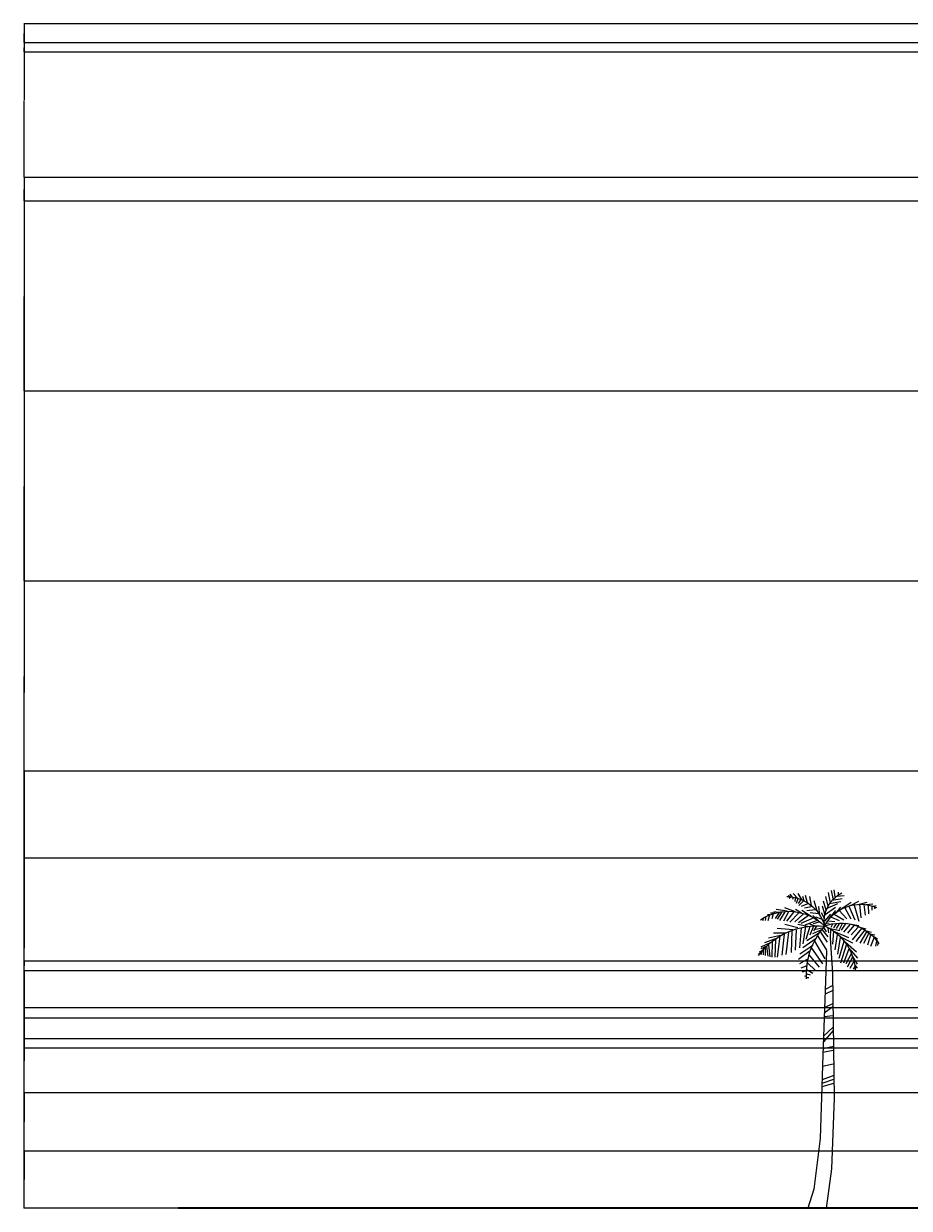
# Model space of a CAD drawing. Units: inches. Extents: x -742 to 1386, y -64 to 951.
# Tile 1 of 8: x -742 to -183, y 106 to 854. Entities that reach past the tile are written whole.
import ezdxf

# ---------------------------------------------------------------- set-up
doc = ezdxf.new("R2010")
doc.units = ezdxf.units.IN
doc.header["$MEASUREMENT"] = 0
for name, color, linetype, lineweight in [('A-ANNO-DIMS', 2, 'Continuous', 18), ('A-ELEV', 7, 'Continuous', 35), ('tree', 3, 'Continuous', 18)]:
    doc.layers.add(name, color=color, linetype=linetype, lineweight=lineweight)
doc.styles.get("Standard").update_dxf_attribs({"font": 'arial.ttf'})
doc.dimstyles.get("Standard").update_dxf_attribs({"dimtxt": 0.18, "dimasz": 0.18, "dimexe": 0.18, "dimexo": 0.0625, "dimgap": 0.09, "dimtad": 0, "dimtih": 1, "dimtoh": 1, "dimdec": 4, "dimzin": 0, "dimdsep": 46, "dimtxsty": 'Standard', "dimcen": 0.09, "dimadec": 0, "dimazin": 0, "dimtfac": 1, "dimtdec": 4, "dimtofl": 0, "dimtmove": 0, "dimatfit": 3, "dimfxl": 1, "dimtolj": 1, "dimtzin": 0, "dimarcsym": 0})

# ---------------------------------------------------------------- blocks, each defined once
blk = doc.blocks.new('*U2')
for p, q in [((-6.727, 197.202), (-11.366, 197.45)), ((-3.441, 194.477), (-10.013, 195.716)), ((-7.5, 199.68), (-7.5, 197.946)), ((-5.567, 196.707), (-4.987, 201.167)), ((-4.407, 195.716), (-3.247, 200.672)), ((-2.474, 193.733), (-1.315, 199.433)), ((-1.121, 190.759), (0.232, 196.955)), ((9.317, 191.255), (10.283, 196.955)), ((11.829, 192.99), (13.182, 197.45)), ((13.956, 194.229), (14.729, 196.955)), ((15.116, 194.477), (17.822, 198.689)), ((16.082, 194.972), (17.822, 192.494)), ((18.015, 195.716), (20.914, 198.689)), ((18.015, 195.468), (18.981, 192.494)), ((19.368, 196.459), (19.948, 193.733)), ((20.914, 196.459), (21.301, 194.972)), ((21.301, 196.459), (22.847, 198.441)), ((22.074, 196.707), (23.427, 195.716)), ((23.234, 196.707), (23.62, 197.698)), ((-29.729, 190.759), (-31.469, 191.255)), ((-30.309, 190.512), (-30.695, 189.025)), ((-25.283, 191.751), (-29.342, 192.246)), ((-28.763, 190.759), (-28.763, 188.281)), ((-26.443, 191.503), (-26.636, 186.051)), ((-20.064, 191.751), (-25.863, 193.238)), ((-23.737, 191.751), (-24.51, 185.06)), ((-21.031, 191.998), (-21.804, 183.325)), ((-15.232, 191.255), (-20.644, 193.981)), ((-17.551, 191.503), (-20.451, 181.343)), ((-14.265, 190.759), (-18.131, 182.086)), ((-9.433, 189.025), (-15.618, 193.238)), ((-11.753, 189.768), (-15.425, 182.83)), ((-8.08, 188.034), (-12.912, 182.83)), ((-1.894, 192.494), (-9.24, 193.733)), ((-6.147, 186.299), (-9.24, 190.264)), ((-0.541, 189.52), (-7.307, 192.494)), ((-5.76, 190.016), (0.618, 185.308)), ((-5.76, 188.034), (-1.508, 182.582)), ((0.038, 188.281), (1.778, 193.981)), ((1.005, 185.803), (2.358, 190.759)), ((4.098, 185.06), (4.678, 190.512)), ((5.837, 187.786), (7.577, 194.229)), ((6.997, 188.529), (12.216, 187.786)), ((8.544, 190.512), (13.763, 189.52)), ((9.51, 184.317), (15.502, 188.034)), ((11.25, 192.494), (15.889, 190.512)), ((14.536, 193.981), (17.242, 191.255)), ((15.695, 186.299), (19.368, 188.777)), ((19.368, 187.29), (26.133, 189.768)), ((20.721, 187.042), (25.167, 181.343)), ((23.814, 187.29), (26.907, 181.343)), ((24.78, 187.538), (31.546, 188.777)), ((26.133, 187.29), (29.419, 181.838)), ((28.066, 187.29), (30.966, 182.582)), ((29.999, 186.795), (33.092, 187.29)), ((-12.332, 180.104), (-9.433, 175.643)), ((-4.987, 185.803), (-10.979, 182.086)), ((-10.206, 180.104), (-8.08, 175.891)), ((-8.273, 180.104), (-6.147, 176.635)), ((-3.247, 183.821), (-8.08, 181.838)), ((-6.34, 179.608), (-4.6, 177.13)), ((-1.315, 181.591), (-5.374, 181.095)), ((-2.668, 185.803), (1.198, 181.343)), ((-0.348, 180.352), (-1.894, 180.104)), ((1.005, 182.582), (2.938, 186.547)), ((2.938, 182.582), (6.61, 183.821)), ((4.098, 180.847), (8.35, 179.608)), ((4.871, 186.051), (10.09, 186.547)), ((4.871, 181.591), (8.544, 184.812)), ((5.644, 181.838), (13.569, 178.865)), ((7.77, 183.325), (16.082, 179.856)), ((11.25, 184.812), (17.628, 180.352)), ((14.536, 185.803), (19.948, 180.847)), ((17.242, 186.547), (23.041, 180.599)), ((29.806, 186.795), (32.319, 183.078)), ((32.512, 186.299), (35.218, 186.299)), ((33.479, 186.051), (34.445, 182.83)), ((35.605, 185.556), (37.151, 185.308)), ((35.798, 185.308), (36.958, 181.591)), ((38.118, 184.317), (38.504, 181.838)), ((39.857, 182.83), (40.244, 181.591)), ((-28.956, 172.174), (-32.435, 170.192)), ((-27.409, 173.413), (-30.695, 172.67)), ((-25.09, 175.148), (-28.376, 174.404)), ((-27.989, 172.422), (-26.056, 166.227)), ((-26.829, 173.661), (-23.544, 167.218)), ((-25.476, 174.652), (-21.224, 167.466)), ((-21.031, 177.626), (-24.897, 176.387)), ((-24.317, 175.891), (-18.711, 168.457)), ((-22.191, 176.635), (-16.391, 169.448)), ((-15.618, 179.36), (-20.644, 178.617)), ((-20.064, 177.626), (-15.812, 172.67)), ((-17.358, 178.617), (-13.299, 173.661)), ((-15.038, 179.36), (-10.786, 174.404)), ((-4.214, 175.148), (-14.072, 170.935)), ((-1.701, 176.882), (-8.66, 175.396)), ((-6.92, 172.917), (-5.374, 163.253)), ((-4.6, 174.9), (-4.021, 166.722)), ((-4.021, 179.36), (-2.861, 177.378)), ((-2.668, 176.387), (-2.376, 170.594)), ((-0.928, 176.882), (-1.508, 173.909)), ((2.551, 175.891), (-0.928, 171.431)), ((3.711, 174.404), (-0.541, 167.961)), ((1.585, 177.13), (0.038, 174.652)), ((1.585, 177.13), (6.61, 176.139)), ((2.938, 175.891), (8.737, 173.413)), ((4.291, 173.909), (12.216, 168.953)), ((6.224, 178.121), (8.157, 175.148)), ((7.384, 178.369), (10.476, 179.36)), ((8.157, 178.121), (10.476, 172.422)), ((10.476, 177.874), (12.796, 169.696)), ((11.829, 177.874), (18.015, 179.113)), ((13.182, 177.874), (14.729, 166.97)), ((15.889, 177.13), (16.855, 164.492)), ((18.015, 177.13), (26.133, 179.113)), ((18.981, 175.891), (19.561, 163.005)), ((20.914, 175.891), (30.966, 176.635)), ((21.688, 175.396), (22.074, 161.518)), ((23.814, 174.404), (25.554, 160.279)), ((25.554, 173.661), (33.285, 173.661)), ((26.52, 173.165), (28.066, 159.784)), ((28.839, 172.174), (36.378, 170.687)), ((-32.628, 167.961), (-33.208, 167.961)), ((-32.628, 167.713), (-32.435, 165.979)), ((-31.082, 169.944), (-32.435, 169.2)), ((-31.662, 168.705), (-31.082, 165.483)), ((-29.922, 170.687), (-27.989, 165.235)), ((-12.139, 167.961), (-19.098, 162.014)), ((-8.466, 171.678), (-16.585, 167.713)), ((-12.719, 166.722), (-9.046, 154.828)), ((-10.979, 168.457), (-7.887, 157.801)), ((-8.853, 170.935), (-7.113, 160.527)), ((5.257, 171.926), (-0.155, 163.005)), ((7.384, 168.705), (0.812, 157.553)), ((6.417, 170.439), (14.729, 164.492)), ((8.544, 165.979), (16.662, 160.527)), ((29.226, 171.926), (30.966, 158.545)), ((30.966, 170.687), (38.891, 167.713)), ((32.126, 169.696), (32.512, 158.545)), ((34.058, 168.705), (34.445, 158.545)), ((35.412, 167.713), (41.404, 164.988)), ((36.378, 166.474), (35.605, 158.792)), ((37.731, 165.235), (36.958, 159.288)), ((37.924, 165.235), (41.404, 163.749)), ((-14.265, 164.244), (-19.678, 158.049)), ((-16.005, 160.031), (-19.484, 154.084)), ((-16.585, 158.545), (-13.106, 152.35)), ((-15.618, 160.775), (-12.332, 154.332)), ((-14.265, 163.749), (-10.786, 154.828)), ((9.317, 164.244), (2.358, 154.332)), ((10.863, 159.784), (4.484, 152.35)), ((10.09, 162.51), (17.435, 157.058)), ((11.443, 157.553), (16.855, 154.332)), ((38.504, 164.492), (38.504, 159.536)), ((39.664, 163.253), (42.37, 161.766)), ((39.857, 162.757), (39.857, 160.031)), ((40.824, 161.766), (41.21, 160.031)), ((41.21, 161.518), (42.757, 160.279)), ((-18.131, 153.589), (-19.484, 151.606)), ((-17.938, 152.597), (-16.972, 151.111)), ((-17.358, 155.819), (-14.845, 151.358)), ((11.829, 155.075), (6.804, 150.119)), ((12.603, 151.111), (8.544, 148.385)), ((12.216, 153.093), (16.082, 151.606)), ((12.603, 149.872), (15.116, 149.128)), ((12.216, 148.137), (10.09, 147.393)), ((12.409, 145.659), (11.056, 145.659)), ((12.409, 146.898), (13.763, 146.402)), ((-4.081, 140.645), (0.753, 138.261)), ((-4.081, 137.547), (0.753, 135.163)), ((-4.081, 129.205), (1.124, 126.821)), ((-4.081, 127.298), (1.31, 123.246)), ((-4.081, 121.578), (1.31, 120.863)), ((-4.453, 112.283), (1.682, 105.133)), ((-4.267, 114.428), (1.682, 108.708)), ((-4.639, 102.273), (1.868, 100.604)), ((-4.453, 99.651), (2.24, 98.459)), ((-4.453, 91.071), (2.426, 89.641)), ((-4.825, 83.921), (2.612, 81.061)), ((-4.639, 81.299), (2.797, 78.916)), ((-4.639, 78.916), (2.797, 76.771))]:
    blk.add_line(p, q)
for points in [[(-2.363, 170.553), (-3.88, 148.505), (-4.988, 69.634), (-3.325, 24.869), (0, 0)], [(-0.116, 162.848), (0.554, 143.532), (2.217, 96.635), (3.88, 44.054), (7.76, 12.079), (11.64, 0)]]:
    blk.add_lwpolyline(points)
for centre, radius, start, end in [((-18.427, 181.448), 19.715, 350.285, 64.11229), ((25.595, 171.567), 25.395, 91.40319, 163.882), ((-21.738, 166.094), 25.899, 27.67115, 112.5305), ((23.687, 155.341), 32.188, 56.19272, 134.3213), ((-9.259, 151.732), 28.386, 68.38311, 147.5322), ((14.394, 148.393), 32.752, 113.7592, 177.4133), ((5.828, 132.718), 45.639, 35.98777, 95.82273), ((-32.8, 147.923), 45.309, 356.1943, 41.37848)]:
    blk.add_arc(centre, radius, start, end)
blk = doc.blocks.new('*D40')
at = {"layer": 'A-ANNO-DIMS', "color": 0, "lineweight": -2, "transparency": 16777216}
for p, q in [((-46.83, 756.74), (-741.55, 756.74)), ((-741.37, 756.56), (-741.37, 431.42)), ((-741.37, 105.92), (-741.37, 431.06)), ((-37.83, 105.74), (-741.55, 105.74))]:
    blk.add_line(p, q, dxfattribs=at)
at = {"layer": 'A-ANNO-DIMS', "color": 0, "transparency": 16777216}
for points in [[(-741.4, 756.56), (-741.34, 756.56), (-741.37, 756.74)], [(-741.4, 105.92), (-741.34, 105.92), (-741.37, 105.74)]]:
    blk.add_solid(points, dxfattribs=at)
at = {"layer": 'Defpoints', "color": 0, "transparency": 16777216}
for p in [(-46.77, 756.74), (-741.37, 105.74), (-37.77, 105.74)]:
    blk.add_point(p, dxfattribs=at)
at = {"layer": 'A-ANNO-DIMS', "color": 0, "transparency": 16777216, "insert": (-741.37, 431.24), "char_height": 0.18, "attachment_point": 5}
blk.add_mtext('\\A1;651', dxfattribs=at)
blk = doc.blocks.new('*D41')
at = {"layer": 'A-ANNO-DIMS', "color": 0, "lineweight": -2, "transparency": 16777216}
for p, q in [((-37.83, 141.74), (-741.55, 141.74)), ((-741.37, 141.56), (-741.37, 123.92)), ((-741.37, 105.92), (-741.37, 123.56)), ((-37.83, 105.74), (-741.55, 105.74))]:
    blk.add_line(p, q, dxfattribs=at)
at = {"layer": 'A-ANNO-DIMS', "color": 0, "transparency": 16777216}
for points in [[(-741.4, 141.56), (-741.34, 141.56), (-741.37, 141.74)], [(-741.4, 105.92), (-741.34, 105.92), (-741.37, 105.74)]]:
    blk.add_solid(points, dxfattribs=at)
at = {"layer": 'Defpoints', "color": 0, "transparency": 16777216}
for p in [(-741.37, 141.74), (-37.77, 141.74), (-37.77, 105.74)]:
    blk.add_point(p, dxfattribs=at)
at = {"layer": 'A-ANNO-DIMS', "color": 0, "transparency": 16777216, "insert": (-741.37, 123.74), "char_height": 0.18, "attachment_point": 5}
blk.add_mtext('\\A1;36', dxfattribs=at)
blk = doc.blocks.new('*D42')
at = {"layer": 'A-ANNO-DIMS', "color": 0, "lineweight": -2, "transparency": 16777216}
for p, q in [((-37.83, 255.74), (-741.55, 255.74)), ((-741.37, 255.56), (-741.37, 198.92)), ((-741.37, 141.92), (-741.37, 198.56)), ((-37.83, 141.74), (-741.55, 141.74))]:
    blk.add_line(p, q, dxfattribs=at)
at = {"layer": 'A-ANNO-DIMS', "color": 0, "transparency": 16777216}
for points in [[(-741.4, 255.56), (-741.34, 255.56), (-741.37, 255.74)], [(-741.4, 141.92), (-741.34, 141.92), (-741.37, 141.74)]]:
    blk.add_solid(points, dxfattribs=at)
at = {"layer": 'Defpoints', "color": 0, "transparency": 16777216}
for p in [(-741.37, 255.74), (-37.77, 255.74), (-37.77, 141.74)]:
    blk.add_point(p, dxfattribs=at)
at = {"layer": 'A-ANNO-DIMS', "color": 0, "transparency": 16777216, "insert": (-741.37, 198.74), "char_height": 0.18, "attachment_point": 5}
blk.add_mtext('\\A1;114', dxfattribs=at)
blk = doc.blocks.new('*D43')
at = {"layer": 'A-ANNO-DIMS', "color": 0, "lineweight": -2, "transparency": 16777216}
for p, q in [((-37.83, 261.74), (-741.55, 261.74)), ((-37.83, 255.74), (-741.55, 255.74)), ((-741.37, 261.56), (-741.37, 258.92)), ((-741.37, 255.92), (-741.37, 258.56))]:
    blk.add_line(p, q, dxfattribs=at)
at = {"layer": 'A-ANNO-DIMS', "color": 0, "transparency": 16777216}
for points in [[(-741.4, 261.56), (-741.34, 261.56), (-741.37, 261.74)], [(-741.4, 255.92), (-741.34, 255.92), (-741.37, 255.74)]]:
    blk.add_solid(points, dxfattribs=at)
at = {"layer": 'Defpoints', "color": 0, "transparency": 16777216}
for p in [(-741.37, 261.74), (-37.77, 261.74), (-37.77, 255.74)]:
    blk.add_point(p, dxfattribs=at)
at = {"layer": 'A-ANNO-DIMS', "color": 0, "transparency": 16777216, "insert": (-741.37, 258.74), "char_height": 0.18, "attachment_point": 5}
blk.add_mtext('\\A1;6', dxfattribs=at)
blk = doc.blocks.new('*D44')
at = {"layer": 'A-ANNO-DIMS', "color": 0, "lineweight": -2, "transparency": 16777216}
for p, q in [((-37.83, 381.74), (-741.55, 381.74)), ((-741.37, 381.56), (-741.37, 321.92)), ((-741.37, 261.92), (-741.37, 321.56)), ((-37.83, 261.74), (-741.55, 261.74))]:
    blk.add_line(p, q, dxfattribs=at)
at = {"layer": 'A-ANNO-DIMS', "color": 0, "transparency": 16777216}
for points in [[(-741.4, 381.56), (-741.34, 381.56), (-741.37, 381.74)], [(-741.4, 261.92), (-741.34, 261.92), (-741.37, 261.74)]]:
    blk.add_solid(points, dxfattribs=at)
at = {"layer": 'Defpoints', "color": 0, "transparency": 16777216}
for p in [(-741.37, 381.74), (-37.77, 381.74), (-37.77, 261.74)]:
    blk.add_point(p, dxfattribs=at)
at = {"layer": 'A-ANNO-DIMS', "color": 0, "transparency": 16777216, "insert": (-741.37, 321.74), "char_height": 0.18, "attachment_point": 5}
blk.add_mtext('\\A1;120', dxfattribs=at)
blk = doc.blocks.new('*D45')
at = {"layer": 'A-ANNO-DIMS', "color": 0, "lineweight": -2, "transparency": 16777216}
for p, q in [((-37.83, 501.74), (-741.55, 501.74)), ((-741.37, 501.56), (-741.37, 441.92)), ((-741.37, 381.92), (-741.37, 441.56)), ((-37.83, 381.74), (-741.55, 381.74))]:
    blk.add_line(p, q, dxfattribs=at)
at = {"layer": 'A-ANNO-DIMS', "color": 0, "transparency": 16777216}
for points in [[(-741.4, 501.56), (-741.34, 501.56), (-741.37, 501.74)], [(-741.4, 381.92), (-741.34, 381.92), (-741.37, 381.74)]]:
    blk.add_solid(points, dxfattribs=at)
at = {"layer": 'Defpoints', "color": 0, "transparency": 16777216}
for p in [(-741.37, 501.74), (-37.77, 501.74), (-37.77, 381.74)]:
    blk.add_point(p, dxfattribs=at)
at = {"layer": 'A-ANNO-DIMS', "color": 0, "transparency": 16777216, "insert": (-741.37, 441.74), "char_height": 0.18, "attachment_point": 5}
blk.add_mtext('\\A1;120', dxfattribs=at)
blk = doc.blocks.new('*D46')
at = {"layer": 'A-ANNO-DIMS', "color": 0, "lineweight": -2, "transparency": 16777216}
for p, q in [((-37.83, 621.74), (-741.55, 621.74)), ((-741.37, 621.56), (-741.37, 561.92)), ((-741.37, 501.92), (-741.37, 561.56)), ((-37.83, 501.74), (-741.55, 501.74))]:
    blk.add_line(p, q, dxfattribs=at)
at = {"layer": 'A-ANNO-DIMS', "color": 0, "transparency": 16777216}
for points in [[(-741.4, 621.56), (-741.34, 621.56), (-741.37, 621.74)], [(-741.4, 501.92), (-741.34, 501.92), (-741.37, 501.74)]]:
    blk.add_solid(points, dxfattribs=at)
at = {"layer": 'Defpoints', "color": 0, "transparency": 16777216}
for p in [(-741.37, 621.74), (-37.77, 621.74), (-37.77, 501.74)]:
    blk.add_point(p, dxfattribs=at)
at = {"layer": 'A-ANNO-DIMS', "color": 0, "transparency": 16777216, "insert": (-741.37, 561.74), "char_height": 0.18, "attachment_point": 5}
blk.add_mtext('\\A1;120', dxfattribs=at)
blk = doc.blocks.new('*D47')
at = {"layer": 'A-ANNO-DIMS', "color": 0, "lineweight": -2, "transparency": 16777216}
for p, q in [((-37.83, 741.74), (-741.55, 741.74)), ((-741.37, 741.56), (-741.37, 681.92)), ((-741.37, 621.92), (-741.37, 681.56)), ((-37.83, 621.74), (-741.55, 621.74))]:
    blk.add_line(p, q, dxfattribs=at)
at = {"layer": 'A-ANNO-DIMS', "color": 0, "transparency": 16777216}
for points in [[(-741.4, 741.56), (-741.34, 741.56), (-741.37, 741.74)], [(-741.4, 621.92), (-741.34, 621.92), (-741.37, 621.74)]]:
    blk.add_solid(points, dxfattribs=at)
at = {"layer": 'Defpoints', "color": 0, "transparency": 16777216}
for p in [(-741.37, 741.74), (-37.77, 741.74), (-37.77, 621.74)]:
    blk.add_point(p, dxfattribs=at)
at = {"layer": 'A-ANNO-DIMS', "color": 0, "transparency": 16777216, "insert": (-741.37, 681.74), "char_height": 0.18, "attachment_point": 5}
blk.add_mtext('\\A1;120', dxfattribs=at)
blk = doc.blocks.new('*D48')
at = {"layer": 'A-ANNO-DIMS', "color": 0, "lineweight": -2, "transparency": 16777216}
for p, q in [((-46.83, 756.74), (-741.55, 756.74)), ((-741.37, 756.56), (-741.37, 749.42)), ((-741.37, 741.92), (-741.37, 749.06)), ((-37.83, 741.74), (-741.55, 741.74))]:
    blk.add_line(p, q, dxfattribs=at)
at = {"layer": 'A-ANNO-DIMS', "color": 0, "transparency": 16777216}
for points in [[(-741.4, 756.56), (-741.34, 756.56), (-741.37, 756.74)], [(-741.4, 741.92), (-741.34, 741.92), (-741.37, 741.74)]]:
    blk.add_solid(points, dxfattribs=at)
at = {"layer": 'Defpoints', "color": 0, "transparency": 16777216}
for p in [(-741.37, 756.74), (-46.77, 756.74), (-37.77, 741.74)]:
    blk.add_point(p, dxfattribs=at)
at = {"layer": 'A-ANNO-DIMS', "color": 0, "transparency": 16777216, "insert": (-741.37, 749.24), "char_height": 0.18, "attachment_point": 5}
blk.add_mtext('\\A1;15', dxfattribs=at)
blk = doc.blocks.new('*D49')
at = {"layer": 'A-ANNO-DIMS', "color": 0, "lineweight": -2, "transparency": 16777216}
for p, q in [((93.05, 178.74), (-741.55, 178.74)), ((-741.37, 178.56), (-741.37, 160.42)), ((-741.37, 141.92), (-741.37, 160.06)), ((46.17, 141.74), (-741.55, 141.74))]:
    blk.add_line(p, q, dxfattribs=at)
at = {"layer": 'A-ANNO-DIMS', "color": 0, "transparency": 16777216}
for points in [[(-741.4, 178.56), (-741.34, 178.56), (-741.37, 178.74)], [(-741.4, 141.92), (-741.34, 141.92), (-741.37, 141.74)]]:
    blk.add_solid(points, dxfattribs=at)
at = {"layer": 'Defpoints', "color": 0, "transparency": 16777216}
for p in [(93.11, 178.74), (-741.37, 141.74), (46.23, 141.74)]:
    blk.add_point(p, dxfattribs=at)
at = {"layer": 'A-ANNO-DIMS', "color": 0, "transparency": 16777216, "insert": (-741.37, 160.24), "char_height": 0.18, "attachment_point": 5}
blk.add_mtext('\\A1;37', dxfattribs=at)
blk = doc.blocks.new('*D50')
at = {"layer": 'A-ANNO-DIMS', "color": 0, "lineweight": -2, "transparency": 16777216}
for p, q in [((84.36, 232.23), (-741.55, 232.23)), ((-741.37, 232.05), (-741.37, 229.16)), ((93.05, 225.74), (-741.55, 225.74)), ((-741.37, 225.92), (-741.37, 228.8))]:
    blk.add_line(p, q, dxfattribs=at)
at = {"layer": 'A-ANNO-DIMS', "color": 0, "transparency": 16777216}
for points in [[(-741.4, 232.05), (-741.34, 232.05), (-741.37, 232.23)], [(-741.4, 225.92), (-741.34, 225.92), (-741.37, 225.74)]]:
    blk.add_solid(points, dxfattribs=at)
at = {"layer": 'Defpoints', "color": 0, "transparency": 16777216}
for p in [(-741.37, 232.23), (84.43, 232.23), (93.11, 225.74)]:
    blk.add_point(p, dxfattribs=at)
at = {"layer": 'A-ANNO-DIMS', "color": 0, "transparency": 16777216, "insert": (-741.37, 228.98), "char_height": 0.18, "attachment_point": 5}
blk.add_mtext('\\A1;6.486', dxfattribs=at)
blk = doc.blocks.new('*D52')
at = {"layer": 'A-ANNO-DIMS', "color": 0, "lineweight": -2, "transparency": 16777216}
for p, q in [((253.17, 853.78), (-741.55, 853.78)), ((-741.37, 853.6), (-741.37, 805.44)), ((-741.37, 756.92), (-741.37, 805.08)), ((262.17, 756.74), (-741.55, 756.74))]:
    blk.add_line(p, q, dxfattribs=at)
at = {"layer": 'A-ANNO-DIMS', "color": 0, "transparency": 16777216}
for points in [[(-741.4, 853.6), (-741.34, 853.6), (-741.37, 853.78)], [(-741.4, 756.92), (-741.34, 756.92), (-741.37, 756.74)]]:
    blk.add_solid(points, dxfattribs=at)
at = {"layer": 'Defpoints', "color": 0, "transparency": 16777216}
for p in [(-741.37, 853.78), (253.23, 853.78), (262.23, 756.74)]:
    blk.add_point(p, dxfattribs=at)
at = {"layer": 'A-ANNO-DIMS', "color": 0, "transparency": 16777216, "insert": (-741.37, 805.26), "char_height": 0.18, "attachment_point": 5}
blk.add_mtext('\\A1;97.04', dxfattribs=at)
blk = doc.blocks.new('*D53')
at = {"layer": 'A-ANNO-DIMS', "color": 0, "lineweight": -2, "transparency": 16777216}
for p, q in [((253.17, 853.78), (-741.55, 853.78)), ((-741.37, 853.6), (-741.37, 847.96)), ((-741.37, 841.96), (-741.37, 847.6)), ((262.17, 841.78), (-741.55, 841.78))]:
    blk.add_line(p, q, dxfattribs=at)
at = {"layer": 'A-ANNO-DIMS', "color": 0, "transparency": 16777216}
for points in [[(-741.4, 853.6), (-741.34, 853.6), (-741.37, 853.78)], [(-741.4, 841.96), (-741.34, 841.96), (-741.37, 841.78)]]:
    blk.add_solid(points, dxfattribs=at)
at = {"layer": 'Defpoints', "color": 0, "transparency": 16777216}
for p in [(253.23, 853.78), (-741.37, 841.78), (262.23, 841.78)]:
    blk.add_point(p, dxfattribs=at)
at = {"layer": 'A-ANNO-DIMS', "color": 0, "transparency": 16777216, "insert": (-741.37, 847.78), "char_height": 0.18, "attachment_point": 5}
blk.add_mtext('\\A1;12', dxfattribs=at)
blk = doc.blocks.new('*D54')
at = {"layer": 'A-ANNO-DIMS', "color": 0, "lineweight": -2, "transparency": 16777216}
for p, q in [((262.17, 841.78), (-741.55, 841.78)), ((-741.37, 841.6), (-741.37, 838.96)), ((-741.37, 835.96), (-741.37, 838.6)), ((262.17, 835.78), (-741.55, 835.78))]:
    blk.add_line(p, q, dxfattribs=at)
at = {"layer": 'A-ANNO-DIMS', "color": 0, "transparency": 16777216}
for points in [[(-741.4, 841.6), (-741.34, 841.6), (-741.37, 841.78)], [(-741.4, 835.96), (-741.34, 835.96), (-741.37, 835.78)]]:
    blk.add_solid(points, dxfattribs=at)
at = {"layer": 'Defpoints', "color": 0, "transparency": 16777216}
for p in [(262.23, 841.78), (-741.37, 835.78), (262.23, 835.78)]:
    blk.add_point(p, dxfattribs=at)
at = {"layer": 'A-ANNO-DIMS', "color": 0, "transparency": 16777216, "insert": (-741.37, 838.78), "char_height": 0.18, "attachment_point": 5}
blk.add_mtext('\\A1;6', dxfattribs=at)
blk = doc.blocks.new('*D55')
at = {"layer": 'A-ANNO-DIMS', "color": 0, "lineweight": -2, "transparency": 16777216}
for p, q in [((295.5, 326.85), (-741.55, 326.85)), ((-741.37, 326.67), (-741.37, 270.04)), ((-741.37, 213.03), (-741.37, 269.67)), ((295.5, 212.85), (-741.55, 212.85))]:
    blk.add_line(p, q, dxfattribs=at)
at = {"layer": 'A-ANNO-DIMS', "color": 0, "transparency": 16777216}
for points in [[(-741.4, 326.67), (-741.34, 326.67), (-741.37, 326.85)], [(-741.4, 213.03), (-741.34, 213.03), (-741.37, 212.85)]]:
    blk.add_solid(points, dxfattribs=at)
at = {"layer": 'Defpoints', "color": 0, "transparency": 16777216}
for p in [(-741.37, 326.85), (295.56, 326.85), (295.56, 212.85)]:
    blk.add_point(p, dxfattribs=at)
at = {"layer": 'A-ANNO-DIMS', "color": 0, "transparency": 16777216, "insert": (-741.37, 269.85), "char_height": 0.18, "attachment_point": 5}
blk.add_mtext('\\A1;114', dxfattribs=at)
blk = doc.blocks.new('*D56')
at = {"layer": 'A-ANNO-DIMS', "color": 0, "lineweight": -2, "transparency": 16777216}
for p, q in [((268.17, 212.85), (-741.55, 212.85)), ((-741.37, 212.67), (-741.37, 210.04)), ((-741.37, 207.03), (-741.37, 209.67)), ((268.17, 206.85), (-741.55, 206.85))]:
    blk.add_line(p, q, dxfattribs=at)
at = {"layer": 'A-ANNO-DIMS', "color": 0, "transparency": 16777216}
for points in [[(-741.4, 212.67), (-741.34, 212.67), (-741.37, 212.85)], [(-741.4, 207.03), (-741.34, 207.03), (-741.37, 206.85)]]:
    blk.add_solid(points, dxfattribs=at)
at = {"layer": 'Defpoints', "color": 0, "transparency": 16777216}
for p in [(-741.37, 212.85), (268.23, 212.85), (268.23, 206.85)]:
    blk.add_point(p, dxfattribs=at)
at = {"layer": 'A-ANNO-DIMS', "color": 0, "transparency": 16777216, "insert": (-741.37, 209.85), "char_height": 0.18, "attachment_point": 5}
blk.add_mtext('\\A1;6', dxfattribs=at)

msp = doc.modelspace()

# ---------------------------------------------------------------- linework, layer by layer
at = {"layer": 'A-ELEV'}
msp.add_line((-37.7724, 105.7399), (-644.1211, 105.7399), dxfattribs=at)

# ---------------------------------------------------------------- block references
at = {"layer": 'tree', "xscale": -1}
msp.add_blockref('*U2', (-235.1265, 105.7399), dxfattribs=at)

# ---------------------------------------------------------------- dimensions: what is measured, and where the dimension line sits
at = {"layer": 'A-ANNO-DIMS'}
for base, p1, p2, override, picture, middle in [((-741.3711, 853.7799), (262.2276, 756.7399), (253.2276, 853.7799), {"dimdec": 2, "dimlfac": 1, "dimrnd": 0, "dimzin": 0, "dimdsep": 46, "dimlunit": 2}, '*D52', (-741.3711, 805.2599)), ((-741.3711, 841.7799), (253.2276, 853.7799), (262.2276, 841.7799), {"dimdec": 0, "dimlfac": 1, "dimrnd": 0, "dimzin": 0, "dimdsep": 46, "dimlunit": 2}, '*D53', (-741.3711, 847.7799)), ((-741.3711, 835.7799), (262.2276, 841.7799), (262.2276, 835.7799), {"dimdec": 0, "dimlfac": 1, "dimrnd": 0, "dimzin": 0, "dimdsep": 46, "dimlunit": 2}, '*D54', (-741.3711, 838.7799)), ((-741.3711, 105.7399), (-46.7724, 756.7399), (-37.7724, 105.7399), {"dimdec": 0, "dimlfac": 1, "dimrnd": 0, "dimzin": 0, "dimdsep": 46, "dimlunit": 2}, '*D40', (-741.3711, 431.2399)), ((-741.3711, 756.7399), (-37.7724, 741.7399), (-46.7724, 756.7399), {"dimdec": 0, "dimlfac": 1, "dimrnd": 0, "dimzin": 0, "dimdsep": 46, "dimlunit": 2}, '*D48', (-741.3711, 749.2399)), ((-741.3711, 741.7399), (-37.7724, 621.7399), (-37.7724, 741.7399), {"dimdec": 0, "dimlfac": 1, "dimrnd": 0, "dimzin": 0, "dimdsep": 46, "dimlunit": 2}, '*D47', (-741.3711, 681.7399)), ((-741.3711, 621.7399), (-37.7724, 501.7399), (-37.7724, 621.7399), {"dimdec": 0, "dimlfac": 1, "dimrnd": 0, "dimzin": 0, "dimdsep": 46, "dimlunit": 2}, '*D46', (-741.3711, 561.7399)), ((-741.3711, 501.7399), (-37.7724, 381.7399), (-37.7724, 501.7399), {"dimdec": 0, "dimlfac": 1, "dimrnd": 0, "dimzin": 0, "dimdsep": 46, "dimlunit": 2}, '*D45', (-741.3711, 441.7399)), ((-741.3711, 381.7399), (-37.7724, 261.7399), (-37.7724, 381.7399), {"dimdec": 0, "dimlfac": 1, "dimrnd": 0, "dimzin": 0, "dimdsep": 46, "dimlunit": 2}, '*D44', (-741.3711, 321.7399)), ((-741.3711, 326.8548), (295.5643, 212.8548), (295.5643, 326.8548), {"dimdec": 0, "dimlfac": 1, "dimrnd": 0, "dimzin": 0, "dimdsep": 46, "dimlunit": 2}, '*D55', (-741.3711, 269.8548)), ((-741.3711, 255.7399), (-37.7724, 141.7399), (-37.7724, 255.7399), {"dimdec": 0, "dimlfac": 1, "dimrnd": 0, "dimzin": 0, "dimdsep": 46, "dimlunit": 2}, '*D42', (-741.3711, 198.7399)), ((-741.3711, 261.7399), (-37.7724, 255.7399), (-37.7724, 261.7399), {"dimdec": 0, "dimlfac": 1, "dimrnd": 0, "dimzin": 0, "dimdsep": 46, "dimlunit": 2}, '*D43', (-741.3711, 258.7399)), ((-741.37107, 232.22544), (93.11175, 225.73986), (84.42625, 232.22544), {"dimdec": 3, "dimlfac": 1, "dimrnd": 0, "dimzin": 0, "dimdsep": 46, "dimlunit": 2}, '*D50', (-741.37107, 228.98265)), ((-741.3711, 212.8548), (268.2276, 206.8548), (268.2276, 212.8548), {"dimdec": 0, "dimlfac": 1, "dimrnd": 0, "dimzin": 0, "dimdsep": 46, "dimlunit": 2}, '*D56', (-741.3711, 209.8548)), ((-741.3711, 141.7399), (93.1117, 178.7399), (46.2276, 141.7399), {"dimdec": 0, "dimlfac": 1, "dimrnd": 0, "dimzin": 0, "dimdsep": 46, "dimlunit": 2}, '*D49', (-741.3711, 160.2399)), ((-741.3711, 141.7399), (-37.7724, 105.7399), (-37.7724, 141.7399), {"dimdec": 0, "dimlfac": 1, "dimrnd": 0, "dimzin": 0, "dimdsep": 46, "dimlunit": 2}, '*D41', (-741.3711, 123.7399))]:
    dim = msp.add_linear_dim(base=base, p1=p1, p2=p2, angle=90, dimstyle='Standard', override=override, dxfattribs=at)
    dim.commit()
    dim.dimension.update_dxf_attribs({"geometry": picture, "text_midpoint": middle})

doc.saveas('drawing.dxf')
